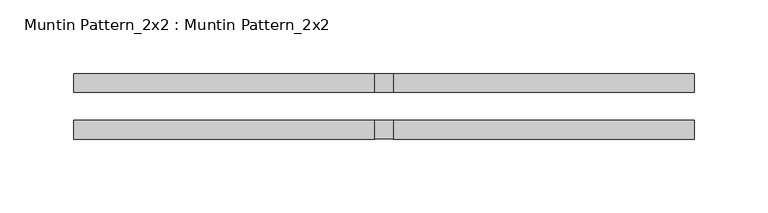
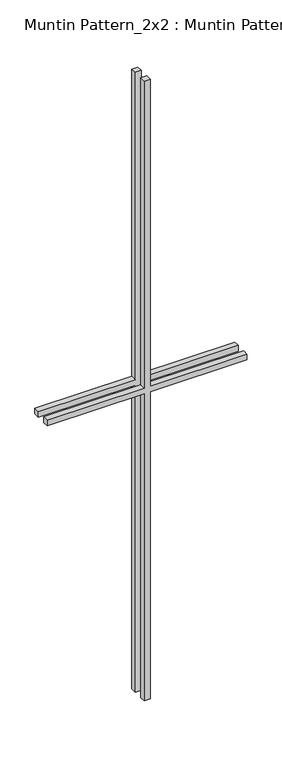
"""IFC4 building model written with IfcOpenShell, lengths in millimetres: proxy geometry, Muntin Pattern_2x2 : Muntin Pattern_2x2."""

from ifc_helpers import new_model, si_unit, frame, origin, place, context, project, spatial, polyline, outline, extrude, source, transform, mapped, element, save


def muntin_pattern_2x2_muntin_pattern_2x2_12159eb8(model_context):
    return source(origin(), model_context, "Body", "SweptSolid", [
        extrude(outline(polyline([(698.5, -6.35), (698.5, -211.1375), (685.8, -211.1375), (685.8, -6.35), (0.0, -6.35), (0.0, 6.35), (685.8, 6.35), (685.8, 211.1375), (698.5, 211.1375), (698.5, 6.35), (1384.3, 6.35), (1384.3, -6.35), (698.5, -6.35)])), frame((0.0, 9.525, 0.0), z_axis=(0.0, 1.0, 0.0), x_axis=(0.0, 0.0, 1.0)), (0.0, 0.0, 1.0), 12.7),
        extrude(outline(polyline([(698.5, -6.35), (698.5, -211.1375), (685.8, -211.1375), (685.8, -6.35), (0.0, -6.35), (0.0, 6.35), (685.8, 6.35), (685.8, 211.1375), (698.5, 211.1375), (698.5, 6.35), (1384.3, 6.35), (1384.3, -6.35), (698.5, -6.35)])), frame((0.0, -22.225, 0.0), z_axis=(0.0, 1.0, 0.0), x_axis=(0.0, 0.0, 1.0)), (0.0, 0.0, 1.0), 12.7),
    ])


if __name__ == "__main__":
    model = new_model("IFC4")
    model_context = context("Model", 3, world=origin())
    ifc_project = project(units=[si_unit("LENGTHUNIT", "METRE", prefix="MILLI")], contexts=[model_context])
    site = spatial("IfcSite", under=ifc_project)
    building = spatial("IfcBuilding", under=site)
    placement = place(None, origin())
    muntin_pattern_2x2_muntin_pattern_2x2_shape = muntin_pattern_2x2_muntin_pattern_2x2_12159eb8(model_context)
    element("IfcBuildingElementProxy", 1, Name="Muntin Pattern_2x2 : Muntin Pattern_2x2", ObjectType="Muntin Pattern_2x2 : Muntin Pattern_2x2", at=placement, inside=building, context=model_context, shape_type="MappedRepresentation", body=[
        mapped(muntin_pattern_2x2_muntin_pattern_2x2_shape, transform((0.0, 0.0, 0.0), x_axis=(1.0, 0.0, 0.0), y_axis=(0.0, 1.0, 0.0), z_axis=(0.0, 0.0, 1.0))),
    ])
    save(model, "model.ifc")

# Revit data of these elements
# Type "Muntin Pattern_2x2 : Muntin Pattern_2x2"
#   Width [instance default] = 4' - 0"
#   Thickness = 0' - 0 1/2"
#   Height [instance default] = 4' - 0"
#   Distance = 0' - 0 3/4"
#   Interior Material [instance default] = none
#   Exterior Material [instance default] = none
#   Default Elevation = 0
# Element 1 (IfcBuildingElementProxy, "Muntin Pattern_2x2 : Muntin Pattern_2x2")
#   Width = 1' - 4 5/8"
#   Height = 4' - 6 1/2"
#   Interior Material = Wood - Stained
#   Exterior Material = Clad - White
#   Materials on its faces: "Clad - White", "Wood - Stained"
# Materials
#   "Clad - White": class "Wood", colour RGB 242 242 238, transparency 0, Cost = 0
#   "Wood - Stained": class "Wood", colour RGB 224 178 126, transparency 0, Cost = 0
